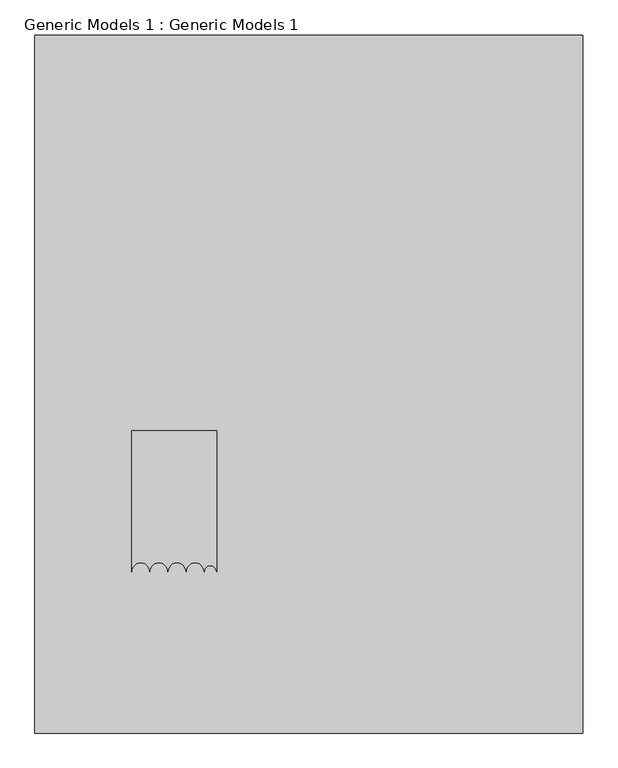
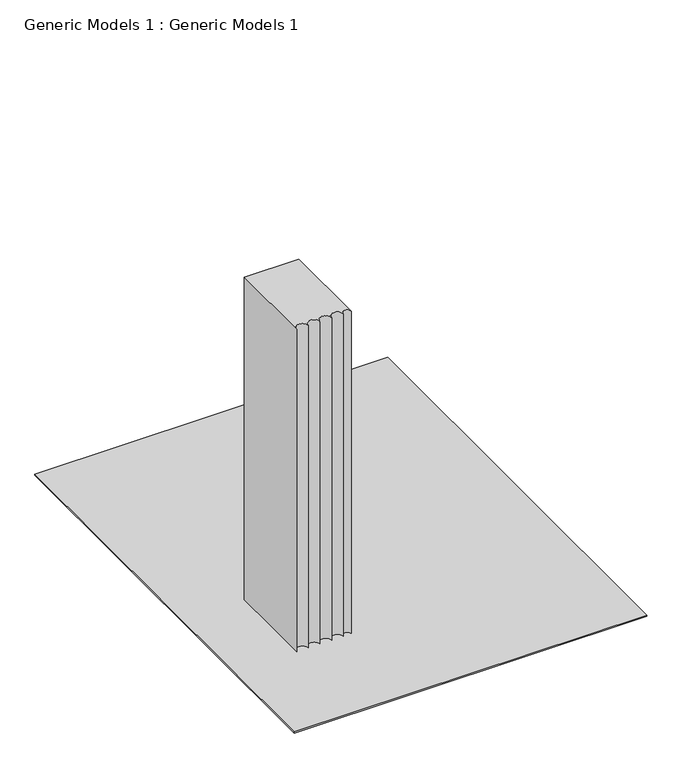
"""IFC4 building model written with IfcOpenShell, lengths in millimetres: proxy geometry, Generic Models 1 : Generic Models 1."""

from ifc_helpers import new_model, si_unit, frame, origin, origin_with_axes, place, context, project, spatial, polyline, circle_curve, outline, extrude, source, transform, mapped, element, save
from ifc_brep_helpers import plane_surface, revolved_surface, advanced_brep


def generic_models_1_generic_models_1_2bf1bac3(model_context):
    return source(origin(), model_context, "Body", "SolidModel", [
        advanced_brep(
        [(-5364.9794854, -5938.7608007, 3352.8), (-5900.364062, -5938.7608007, 3352.8), (-5900.364062, -6829.6142637, 3352.8), (-5786.064062, -6829.6142637, 3352.8), (-5671.764062, -6829.6142637, 3352.8), (-5557.464062, -6829.6142637, 3352.8), (-5443.164062, -6829.6142637, 3352.8), (-5364.9794854, -6829.6142637, 3352.8), (-5364.9794854, -5938.7608007, 12.0054688), (-5364.9794854, -6829.6142637, 12.0054688), (-5443.164062, -6829.6142637, 12.0054688), (-5557.464062, -6829.6142637, 12.0054688), (-5671.764062, -6829.6142637, 12.0054688), (-5786.064062, -6829.6142637, 12.0054688), (-5900.364062, -6829.6142637, 12.0054688), (-5900.364062, -5938.7608007, 12.0054688)],
        [
            (0, 1),
            (1, 2),
            (2, 3, circle_curve(frame((-5843.214062, -6829.6142637, 3352.8), z_axis=(0.0, 0.0, -1.0), x_axis=(-1.0, 0.0, 0.0)), 57.15)),
            (3, 4, circle_curve(frame((-5728.914062, -6829.6142637, 3352.8), z_axis=(0.0, 0.0, -1.0), x_axis=(-1.0, 0.0, 0.0)), 57.15)),
            (4, 5, circle_curve(frame((-5614.614062, -6829.6142637, 3352.8), z_axis=(0.0, 0.0, -1.0), x_axis=(-1.0, 0.0, 0.0)), 57.15)),
            (5, 6, circle_curve(frame((-5500.314062, -6829.6142637, 3352.8), z_axis=(0.0, 0.0, -1.0), x_axis=(-1.0, 0.0, 0.0)), 57.15)),
            (6, 7, circle_curve(frame((-5404.0717737, -6829.6142637, 3352.8), z_axis=(0.0, 0.0, -1.0), x_axis=(-1.0, 0.0, 0.0)), 39.0922883)),
            (7, 0),
            (8, 9),
            (9, 10, circle_curve(frame((-5404.0717737, -6829.6142637, 12.0054688), z_axis=(0.0, 0.0, 1.0), x_axis=(-1.0, 0.0, 0.0)), 39.0922883)),
            (10, 11, circle_curve(frame((-5500.314062, -6829.6142637, 12.0054688), z_axis=(0.0, 0.0, 1.0), x_axis=(-1.0, 0.0, 0.0)), 57.15)),
            (11, 12, circle_curve(frame((-5614.614062, -6829.6142637, 12.0054688), z_axis=(0.0, 0.0, 1.0), x_axis=(-1.0, 0.0, 0.0)), 57.15)),
            (12, 13, circle_curve(frame((-5728.914062, -6829.6142637, 12.0054688), z_axis=(0.0, 0.0, 1.0), x_axis=(-1.0, 0.0, 0.0)), 57.15)),
            (13, 14, circle_curve(frame((-5843.214062, -6829.6142637, 12.0054688), z_axis=(0.0, 0.0, 1.0), x_axis=(-1.0, 0.0, 0.0)), 57.15)),
            (14, 15),
            (15, 8),
            (0, 8),
            (15, 1),
            (14, 2),
            (13, 3),
            (12, 4),
            (11, 5),
            (10, 6),
            (9, 7),
        ],
        [
            plane_surface(frame((-5900.364062, -5938.7608007, 3352.8), z_axis=(0.0, 0.0, 1.0), x_axis=(-1.0, 0.0, 0.0))),
            plane_surface(frame((-5900.364062, -5938.7608007, 12.0054688), z_axis=(0.0, 0.0, -1.0), x_axis=(1.0, 0.0, 0.0))),
            plane_surface(frame((-5364.9794854, -5938.7608007, 3352.8), z_axis=(0.0, 1.0, 0.0), x_axis=(0.0, 0.0, -1.0))),
            plane_surface(frame((-5900.364062, -5938.7608007, 3352.8), z_axis=(-1.0, 0.0, 0.0), x_axis=(0.0, 0.0, -1.0))),
            revolved_surface(polyline([(-5900.364062, -6829.6142637, 12.0054688), (-5900.364062, -6829.6142637, 3352.8)]), (-5843.214062, -6829.6142637, 12.0054688), (0.0, 0.0, -1.0)),
            revolved_surface(polyline([(-5786.0640619999995, -6829.6142637, 12.0054688), (-5786.0640619999995, -6829.6142637, 3352.8)]), (-5728.914062, -6829.6142637, 12.0054688), (0.0, 0.0, -1.0)),
            revolved_surface(polyline([(-5671.764061999999, -6829.6142637, 12.0054688), (-5671.764061999999, -6829.6142637, 3352.8)]), (-5614.614062, -6829.6142637, 12.0054688), (0.0, 0.0, -1.0)),
            revolved_surface(polyline([(-5557.464062, -6829.6142637, 12.0054688), (-5557.464062, -6829.6142637, 3352.8)]), (-5500.314062, -6829.6142637, 12.0054688), (0.0, 0.0, -1.0)),
            revolved_surface(polyline([(-5443.164062000001, -6829.6142637, 12.0054688), (-5443.164062000001, -6829.6142637, 3352.8)]), (-5404.0717737, -6829.6142637, 12.0054688), (0.0, 0.0, -1.0)),
            plane_surface(frame((-5364.9794854, -6829.6142637, 3352.8), z_axis=(1.0, 0.0, 0.0), x_axis=(0.0, 0.0, -1.0))),
        ],
        [
            (0, [[1, 2, 3, 4, 5, 6, 7, 8]]),
            (1, [[9, 10, 11, 12, 13, 14, 15, 16]]),
            (2, [[-1, 17, -16, 18]]),
            (3, [[-2, -18, -15, 19]]),
            (4, [[-3, -19, -14, 20]]),
            (5, [[-4, -20, -13, 21]]),
            (6, [[-5, -21, -12, 22]]),
            (7, [[-6, -22, -11, 23]]),
            (8, [[-7, -23, -10, 24]]),
            (9, [[-8, -24, -9, -17]]),
        ],
    ),
        extrude(outline(polyline([(-3055.564062, -3444.8082297), (-3055.564062, -7845.6142637), (-6509.964062, -7845.6142637), (-6509.964062, -3444.8082297), (-3055.564062, -3444.8082297)])), origin_with_axes(), (0.0, 0.0, 1.0), 12.0054688),
    ])


if __name__ == "__main__":
    model = new_model("IFC4")
    model_context = context("Model", 3, world=origin())
    ifc_project = project(units=[si_unit("LENGTHUNIT", "METRE", prefix="MILLI")], contexts=[model_context])
    site = spatial("IfcSite", under=ifc_project)
    building = spatial("IfcBuilding", under=site)
    placement = place(None, origin())
    generic_models_1_generic_models_1_shape = generic_models_1_generic_models_1_2bf1bac3(model_context)
    element("IfcBuildingElementProxy", 1, Name="Generic Models 1 : Generic Models 1", ObjectType="Generic Models 1 : Generic Models 1", at=placement, inside=building, context=model_context, shape_type="MappedRepresentation", body=[
        mapped(generic_models_1_generic_models_1_shape, transform((0.0, 0.0, 0.0), x_axis=(1.0, 0.0, 0.0), y_axis=(0.0, 1.0, 0.0), z_axis=(0.0, 0.0, 1.0))),
    ])
    save(model, "model.ifc")

# Revit data of these elements
# Element 1 (IfcBuildingElementProxy, "Generic Models 1 : Generic Models 1")
#   Materials on its faces: "FLOOR TILES", "BURGUNDY COLOUR", "LIVING ROOM WALL"
# Materials
#   "FLOOR TILES": class "Generic", colour RGB 120 120 120, transparency 0, Cost = 0
#   "BURGUNDY COLOUR": class "Generic", colour RGB 120 120 120, transparency 0, Cost = 0
#   "LIVING ROOM WALL": class "Generic", colour RGB 120 120 120, transparency 0, Cost = 0
